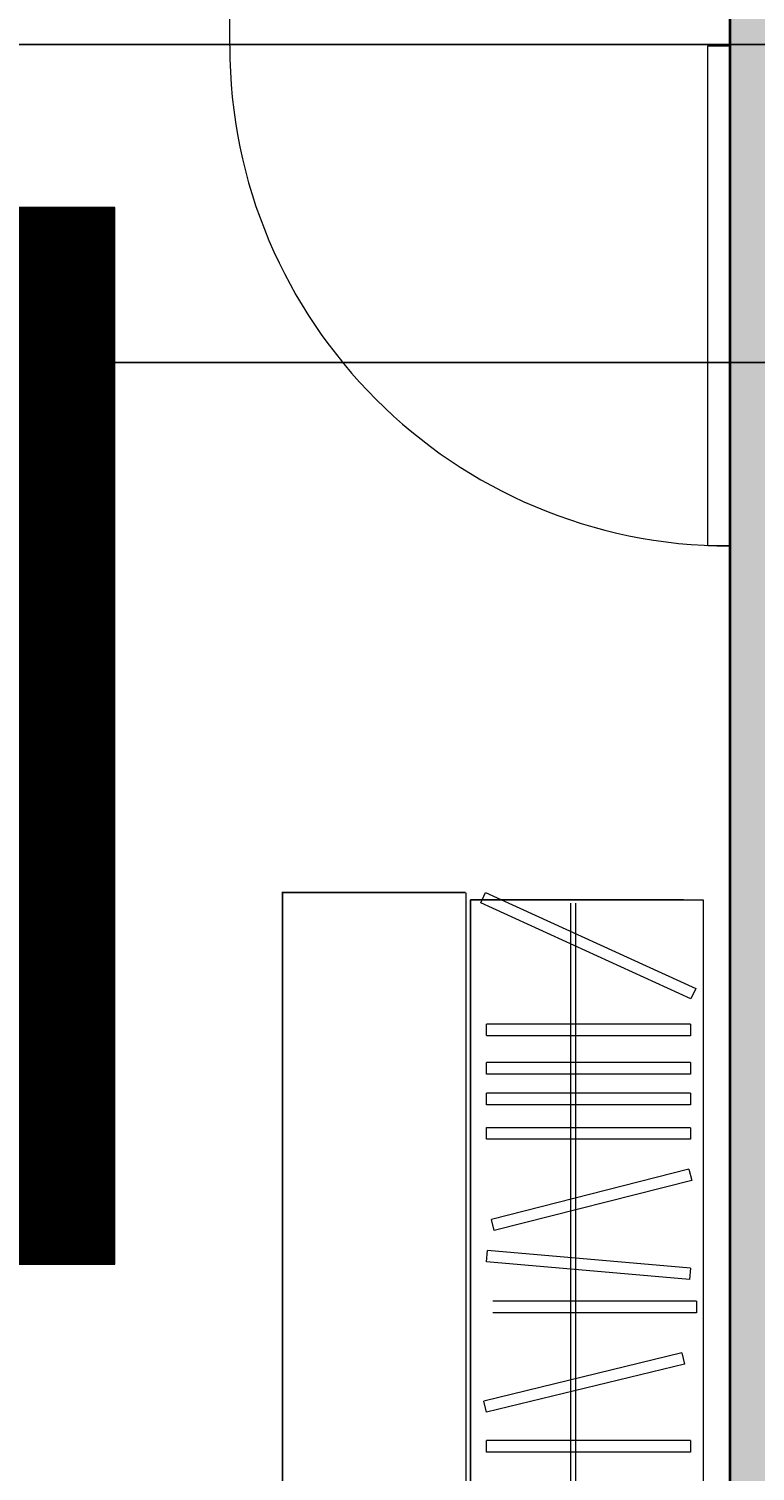
# Model space of a CAD drawing. Units: inches. Extents: x 192 to 1361, y -1362 to 367.
# Tile 9 of 23: x 495 to 649, y -761 to -454. Entities that reach past the tile are written whole.
import ezdxf

# ---------------------------------------------------------------- set-up
doc = ezdxf.new("R2010")
doc.units = ezdxf.units.IN
doc.header["$MEASUREMENT"] = 0
for name, color, linetype, lineweight in [('A-ANNO-DIMS', 2, 'Continuous', 18), ('A-DOOR', 4, 'Continuous', 18), ('A-FLOR', 8, 'Continuous', 18), ('A-WALL-PATT', 250, 'Continuous', 13), ('closet', 32, 'Continuous', 18), ('walls', 7, 'Continuous', 35)]:
    doc.layers.add(name, color=color, linetype=linetype, lineweight=lineweight)
doc.layers.add('A-FLOR-PATT', color=254, linetype='Continuous', lineweight=13, true_color=0xfeeab9)
doc.styles.get("Standard").update_dxf_attribs({"font": 'arial.ttf'})
doc.dimstyles.get("Standard").update_dxf_attribs({"dimtxt": 0.18, "dimasz": 0.18, "dimexe": 0.18, "dimexo": 0.0625, "dimgap": 0.09, "dimtad": 0, "dimtih": 1, "dimtoh": 1, "dimzin": 0, "dimdsep": 46, "dimlunit": 3, "dimtxsty": 'Standard', "dimcen": 0.09, "dimadec": 0, "dimazin": 0, "dimtfac": 1, "dimtofl": 0, "dimtmove": 0, "dimatfit": 3, "dimfxl": 1, "dimtolj": 1, "dimtzin": 0, "dimarcsym": 0})

# ---------------------------------------------------------------- blocks, each defined once
blk = doc.blocks.new('*U2')
for p, q in [((0, 0), (0, -6)), ((40, 0), (40, -6))]:
    blk.add_line(p, q)
blk.add_lwpolyline([(0, 0), (0, 40), (1.75, 40), (1.75, 0)], close=True)
blk.add_arc((0, 0), 40, 0, 90)
blk = doc.blocks.new('closet')
at = {"layer": 'closet'}
for p, q in [((-0.712, -5.577), (5.592, 8.191)), ((6.268, 7.882), (-0.036, -5.886)), ((5.592, 8.191), (6.268, 7.882)), ((7.922, 7.842), (8.679, 7.842)), ((7.922, 7.842), (7.922, -5.515)), ((8.679, 7.842), (8.679, -5.515)), ((10.443, 7.842), (11.2, 7.842)), ((10.443, 7.842), (10.443, -5.515)), ((11.2, 7.842), (11.2, -5.515)), ((12.449, 7.842), (13.206, 7.842)), ((12.449, 7.842), (12.449, -5.515)), ((13.206, 7.842), (13.206, -5.515)), ((14.712, 7.842), (15.469, 7.842)), ((14.712, 7.842), (14.712, -5.515)), ((15.469, 7.842), (15.469, -5.515)), ((17.436, 7.748), (18.17, 7.935)), ((17.436, 7.748), (20.729, -5.196)), ((18.17, 7.935), (21.462, -5.009)), ((23.918, 7.842), (22.755, -5.464)), ((24.672, 7.776), (23.509, -5.53)), ((23.918, 7.842), (24.672, 7.776)), ((26.086, 8.254), (26.086, -5.103)), ((26.843, 8.254), (26.843, -5.103)), ((35.229, 7.842), (35.229, -5.515)), ((35.986, 7.842), (35.986, -5.515)), ((40.326, 7.842), (40.326, -5.515)), ((41.083, 7.842), (41.083, -5.515)), ((42.848, 7.842), (42.848, -5.515)), ((43.605, 7.842), (43.605, -5.515)), ((45.896, 7.842), (45.896, -5.515)), ((46.653, 7.842), (46.653, -5.515)), ((50.066, 7.842), (50.066, -5.515)), ((50.823, 7.842), (50.823, -5.515)), ((53.325, 7.842), (53.325, -5.515)), ((54.081, 7.842), (54.081, -5.515)), ((55.896, 7.842), (55.896, -5.515)), ((56.653, 7.842), (56.653, -5.515)), ((57.994, -5.577), (64.297, 8.191)), ((64.973, 7.882), (58.669, -5.886)), ((60.189, -5.577), (66.493, 8.191)), ((67.169, 7.882), (60.865, -5.886)), ((61.999, -5.577), (68.303, 8.191)), ((68.978, 7.882), (62.675, -5.886)), ((69.963, 7.842), (69.963, -5.515)), ((70.72, 7.842), (70.72, -5.515)), ((72.429, 7.842), (72.429, -5.515)), ((73.186, 7.842), (73.186, -5.515)), ((74.817, 7.842), (74.817, -5.515)), ((75.574, 7.842), (75.574, -5.515)), ((76.936, 7.842), (76.936, -5.515)), ((77.693, 7.842), (77.693, -5.515)), ((-0.232, 7.394), (-0.232, -6.566)), ((29.485, 7.286), (32.636, -5.694)), ((30.221, 7.465), (33.372, -5.515)), ((56.234, 0.335), (0, 0.335)), ((56.2, 0), (0, 0)), ((56.2, 0), (78.757, 0)), ((56.234, 0.335), (78.757, 0.335)), ((-0.036, -5.886), (-0.712, -5.577)), ((21.462, -5.009), (20.729, -5.196)), ((23.509, -5.53), (22.755, -5.464)), ((33.372, -5.515), (32.636, -5.694)), ((35.986, -5.515), (35.229, -5.515)), ((41.083, -5.515), (40.326, -5.515)), ((43.605, -5.515), (42.848, -5.515)), ((46.653, -5.515), (45.896, -5.515)), ((50.823, -5.515), (50.066, -5.515)), ((54.081, -5.515), (53.325, -5.515)), ((56.653, -5.515), (55.896, -5.515)), ((58.669, -5.886), (57.994, -5.577)), ((60.865, -5.886), (60.189, -5.577)), ((62.675, -5.886), (61.999, -5.577)), ((70.72, -5.515), (69.963, -5.515)), ((73.186, -5.515), (72.429, -5.515)), ((75.574, -5.515), (74.817, -5.515)), ((77.693, -5.515), (76.936, -5.515))]:
    blk.add_line(p, q, dxfattribs=at)
blk = doc.blocks.new('rotated closet')
at = {"layer": 'closet'}
for p, q in [((26.318, 0.86), (27.074, 0.86)), ((29.717, -0.108), (30.452, 0.071)), ((35.461, 0.448), (36.217, 0.448)), ((40.558, 0.448), (41.314, 0.448)), ((43.08, 0.448), (43.837, 0.448)), ((46.128, 0.448), (46.884, 0.448)), ((50.298, 0.448), (51.055, 0.448)), ((53.556, 0.448), (54.313, 0.448)), ((56.128, 0.448), (56.884, 0.448)), ((64.529, 0.797), (65.205, 0.488)), ((66.725, 0.797), (67.4, 0.488)), ((68.534, 0.797), (69.21, 0.488)), ((70.195, 0.448), (70.952, 0.448)), ((72.66, 0.448), (73.417, 0.448)), ((75.049, 0.448), (75.806, 0.448)), ((77.168, 0.448), (77.924, 0.448)), ((78.989, 0), (78.989, -13.96)), ((8.91, -12.909), (8.153, -12.909)), ((11.431, -12.909), (10.675, -12.909)), ((13.437, -12.909), (12.681, -12.909)), ((15.7, -12.909), (14.943, -12.909)), ((0, -13.96), (78.989, -13.96)), ((-0.456, -14.274), (79.544, -14.274))]:
    blk.add_line(p, q, dxfattribs=at)
blk.add_blockref('closet', (0.232, -7.394), dxfattribs=at)
blk = doc.blocks.new('*D31')
at = {"layer": 'A-ANNO-DIMS', "color": 0, "lineweight": -2, "transparency": 16777216}
for p, q in [((587.7, -637.86), (548.65, -637.86)), ((548.83, -638.04), (548.83, -767.46)), ((548.83, -897.24), (548.83, -767.83)), ((587.7, -897.42), (548.65, -897.42))]:
    blk.add_line(p, q, dxfattribs=at)
at = {"layer": 'A-ANNO-DIMS', "color": 0, "transparency": 16777216}
for points in [[(548.8, -638.04), (548.86, -638.04), (548.83, -637.86)], [(548.8, -897.24), (548.86, -897.24), (548.83, -897.42)]]:
    blk.add_solid(points, dxfattribs=at)
at = {"layer": 'Defpoints', "color": 0, "transparency": 16777216}
for p in [(587.76, -637.86), (548.83, -897.42), (587.76, -897.42)]:
    blk.add_point(p, dxfattribs=at)
at = {"layer": 'A-ANNO-DIMS', "color": 0, "transparency": 16777216, "insert": (548.83, -767.64), "char_height": 0.18, "attachment_point": 5}
blk.add_mtext('\\A1;WARDROBE 260', dxfattribs=at)
blk = doc.blocks.new('*D69')
at = {"layer": 'A-ANNO-DIMS', "color": 0, "lineweight": -2, "transparency": 16777216}
for p, q in [((981.75, -457.5), (192.16, -457.5)), ((192.34, -457.68), (192.34, -491.13)), ((192.34, -524.95), (192.34, -491.5)), ((980.52, -525.13), (192.16, -525.13))]:
    blk.add_line(p, q, dxfattribs=at)
at = {"layer": 'A-ANNO-DIMS', "color": 0, "transparency": 16777216}
for points in [[(192.31, -457.68), (192.37, -457.68), (192.34, -457.5)], [(192.31, -524.95), (192.37, -524.95), (192.34, -525.13)]]:
    blk.add_solid(points, dxfattribs=at)
at = {"layer": 'Defpoints', "color": 0, "transparency": 16777216}
for p in [(981.81, -457.5), (192.34, -525.13), (980.58, -525.13)]:
    blk.add_point(p, dxfattribs=at)
at = {"layer": 'A-ANNO-DIMS', "color": 0, "transparency": 16777216, "insert": (192.34, -491.31), "char_height": 0.18, "attachment_point": 5}
blk.add_mtext('\\A1;67.63', dxfattribs=at)

msp = doc.modelspace()

# ---------------------------------------------------------------- hatches: boundary and pattern name
at = {"layer": 'A-FLOR-PATT'}
h = msp.add_hatch(dxfattribs=at)
h.set_pattern_fill('ANSI31', color=256)
edge = h.paths.add_edge_path()
edge.add_line((513.1511, -492.1899), (327.1032, -492.1899))
edge.add_line((327.1032, -492.1899), (327.1032, -508.439))
edge.add_line((327.1032, -508.439), (326.9465, -508.439))
edge.add_line((326.9465, -508.439), (326.6697, -537.1419))
edge.add_line((326.6697, -537.1419), (391.8439, -537.1419))
edge.add_line((391.8439, -537.1419), (391.8439, -520.2026))
edge.add_line((391.8439, -520.2026), (393.0084, -520.2026))
edge.add_spline(control_points=[(393.2858, -517.1545), (392.9584, -517.4172), (392.3119, -517.936), (392.9583, -518.8629), (393.4257, -519.6151), (393.1386, -520.0192), (393.0084, -520.2026)], knot_values=[0, 0, 0, 0, 0.65327829, 1.2901376, 1.74045698, 2.11445126, 2.11445126, 2.11445126, 2.11445126], degree=3, periodic=0)
edge.add_line((393.0084, -520.2026), (395.1098, -520.2026))
edge.add_spline(control_points=[(395.3872, -517.1545), (395.0598, -517.4172), (394.4133, -517.936), (395.0598, -518.8629), (395.5272, -519.6151), (395.2401, -520.0192), (395.1098, -520.2026)], knot_values=[0, 0, 0, 0, 0.65327829, 1.2901376, 1.74045698, 2.11445126, 2.11445126, 2.11445126, 2.11445126], degree=3, periodic=0)
edge.add_line((395.1098, -520.2026), (397.3144, -520.2026))
edge.add_spline(control_points=[(397.5918, -517.1545), (397.2644, -517.4172), (396.6179, -517.936), (397.2643, -518.8629), (397.7317, -519.6151), (397.4446, -520.0192), (397.3144, -520.2026)], knot_values=[0, 0, 0, 0, 0.65327829, 1.2901376, 1.74045698, 2.11445126, 2.11445126, 2.11445126, 2.11445126], degree=3, periodic=0)
edge.add_line((397.3144, -520.2026), (399.2806, -520.2026))
edge.add_spline(control_points=[(399.558, -517.1545), (399.2307, -517.4172), (398.5841, -517.936), (399.2306, -518.8629), (399.698, -519.6151), (399.4109, -520.0192), (399.2806, -520.2026)], knot_values=[0, 0, 0, 0, 0.65327829, 1.2901376, 1.74045698, 2.11445126, 2.11445126, 2.11445126, 2.11445126], degree=3, periodic=0)
edge.add_line((399.2806, -520.2026), (401.664, -520.2026))
edge.add_spline(control_points=[(401.9414, -517.1545), (401.614, -517.4172), (400.9675, -517.936), (401.6139, -518.8629), (402.0814, -519.6151), (401.7943, -520.0192), (401.664, -520.2026)], knot_values=[0, 0, 0, 0, 0.65327829, 1.2901376, 1.74045698, 2.11445126, 2.11445126, 2.11445126, 2.11445126], degree=3, periodic=0)
edge.add_line((401.664, -520.2026), (403.6961, -520.2026))
edge.add_spline(control_points=[(403.9735, -517.1545), (403.6461, -517.4172), (402.9996, -517.936), (403.6461, -518.8629), (404.1135, -519.6151), (403.8264, -520.0192), (403.6961, -520.2026)], knot_values=[0, 0, 0, 0, 0.65327829, 1.2901376, 1.74045698, 2.11445126, 2.11445126, 2.11445126, 2.11445126], degree=3, periodic=0)
edge.add_line((403.6961, -520.2026), (405.6624, -520.2026))
edge.add_spline(control_points=[(405.9398, -517.1545), (405.6124, -517.4172), (404.9659, -517.936), (405.6123, -518.8629), (406.0797, -519.6151), (405.7926, -520.0192), (405.6624, -520.2026)], knot_values=[0, 0, 0, 0, 0.65327829, 1.2901376, 1.74045698, 2.11445126, 2.11445126, 2.11445126, 2.11445126], degree=3, periodic=0)
edge.add_line((405.6624, -520.2026), (408.0457, -520.2026))
edge.add_spline(control_points=[(408.3231, -517.1545), (407.9958, -517.4172), (407.3493, -517.936), (407.9957, -518.8629), (408.4631, -519.6151), (408.176, -520.0192), (408.0457, -520.2026)], knot_values=[0, 0, 0, 0, 0.65327829, 1.2901376, 1.74045698, 2.11445126, 2.11445126, 2.11445126, 2.11445126], degree=3, periodic=0)
edge.add_line((408.0457, -520.2026), (410.8462, -520.2026))
edge.add_spline(control_points=[(411.1236, -517.1545), (410.7962, -517.4172), (410.1497, -517.936), (410.7961, -518.8629), (411.2635, -519.6151), (410.9764, -520.0192), (410.8462, -520.2026)], knot_values=[0, 0, 0, 0, 0.65327829, 1.2901376, 1.74045698, 2.11445126, 2.11445126, 2.11445126, 2.11445126], degree=3, periodic=0)
edge.add_line((410.8462, -520.2026), (413.2295, -520.2026))
edge.add_spline(control_points=[(413.5069, -517.1545), (413.1795, -517.4172), (412.533, -517.936), (413.1794, -518.8629), (413.6468, -519.6151), (413.3597, -520.0192), (413.2295, -520.2026)], knot_values=[0, 0, 0, 0, 0.65327829, 1.2901376, 1.74045698, 2.11445126, 2.11445126, 2.11445126, 2.11445126], degree=3, periodic=0)
edge.add_line((413.2295, -520.2026), (415.434, -520.2026))
edge.add_spline(control_points=[(415.7114, -517.1545), (415.3841, -517.4172), (414.7376, -517.936), (415.384, -518.8629), (415.8514, -519.6151), (415.5643, -520.0192), (415.434, -520.2026)], knot_values=[0, 0, 0, 0, 0.65327829, 1.2901376, 1.74045698, 2.11445126, 2.11445126, 2.11445126, 2.11445126], degree=3, periodic=0)
edge.add_line((415.434, -520.2026), (417.5321, -520.2026))
edge.add_spline(control_points=[(417.8095, -517.1545), (417.4821, -517.4172), (416.8356, -517.936), (417.482, -518.8629), (417.9494, -519.6151), (417.6623, -520.0192), (417.5321, -520.2026)], knot_values=[0, 0, 0, 0, 0.65327829, 1.2901376, 1.74045698, 2.11445126, 2.11445126, 2.11445126, 2.11445126], degree=3, periodic=0)
edge.add_line((417.5321, -520.2026), (419.7366, -520.2026))
edge.add_spline(control_points=[(420.014, -517.1545), (419.6867, -517.4172), (419.0401, -517.936), (419.6866, -518.8629), (420.154, -519.6151), (419.8669, -520.0192), (419.7366, -520.2026)], knot_values=[0, 0, 0, 0, 0.65327829, 1.2901376, 1.74045698, 2.11445126, 2.11445126, 2.11445126, 2.11445126], degree=3, periodic=0)
edge.add_line((419.7366, -520.2026), (421.7029, -520.2026))
edge.add_spline(control_points=[(421.9803, -517.1545), (421.6529, -517.4172), (421.0064, -517.936), (421.6528, -518.8629), (422.1202, -519.6151), (421.8331, -520.0192), (421.7029, -520.2026)], knot_values=[0, 0, 0, 0, 0.65327829, 1.2901376, 1.74045698, 2.11445126, 2.11445126, 2.11445126, 2.11445126], degree=3, periodic=0)
edge.add_line((421.7029, -520.2026), (424.0863, -520.2026))
edge.add_spline(control_points=[(424.3637, -517.1545), (424.0363, -517.4172), (423.3898, -517.936), (424.0362, -518.8629), (424.5036, -519.6151), (424.2165, -520.0192), (424.0863, -520.2026)], knot_values=[0, 0, 0, 0, 0.65327829, 1.2901376, 1.74045698, 2.11445126, 2.11445126, 2.11445126, 2.11445126], degree=3, periodic=0)
edge.add_line((424.0863, -520.2026), (426.1184, -520.2026))
edge.add_spline(control_points=[(426.3958, -517.1545), (426.0684, -517.4172), (425.4219, -517.936), (426.0683, -518.8629), (426.5357, -519.6151), (426.2486, -520.0192), (426.1184, -520.2026)], knot_values=[0, 0, 0, 0, 0.65327829, 1.2901376, 1.74045698, 2.11445126, 2.11445126, 2.11445126, 2.11445126], degree=3, periodic=0)
edge.add_line((426.1184, -520.2026), (428.0846, -520.2026))
edge.add_spline(control_points=[(428.362, -517.1545), (428.0346, -517.4172), (427.3881, -517.936), (428.0346, -518.8629), (428.502, -519.6151), (428.2149, -520.0192), (428.0846, -520.2026)], knot_values=[0, 0, 0, 0, 0.65327829, 1.2901376, 1.74045698, 2.11445126, 2.11445126, 2.11445126, 2.11445126], degree=3, periodic=0)
edge.add_line((428.0846, -520.2026), (430.468, -520.2026))
edge.add_spline(control_points=[(430.7454, -517.1545), (430.418, -517.4172), (429.7715, -517.936), (430.4179, -518.8629), (430.8853, -519.6151), (430.5983, -520.0192), (430.468, -520.2026)], knot_values=[0, 0, 0, 0, 0.65327829, 1.2901376, 1.74045698, 2.11445126, 2.11445126, 2.11445126, 2.11445126], degree=3, periodic=0)
edge.add_line((430.468, -520.2026), (433.2684, -520.2026))
edge.add_spline(control_points=[(433.5458, -517.1545), (433.2184, -517.4172), (432.5719, -517.936), (433.2184, -518.8629), (433.6858, -519.6151), (433.3987, -520.0192), (433.2684, -520.2026)], knot_values=[0, 0, 0, 0, 0.65327829, 1.2901376, 1.74045698, 2.11445126, 2.11445126, 2.11445126, 2.11445126], degree=3, periodic=0)
edge.add_line((433.2684, -520.2026), (435.6517, -520.2026))
edge.add_spline(control_points=[(435.9291, -517.1545), (435.6017, -517.4172), (434.9552, -517.936), (435.6017, -518.8629), (436.0691, -519.6151), (435.782, -520.0192), (435.6517, -520.2026)], knot_values=[0, 0, 0, 0, 0.65327829, 1.2901376, 1.74045698, 2.11445126, 2.11445126, 2.11445126, 2.11445126], degree=3, periodic=0)
edge.add_line((435.6517, -520.2026), (437.8563, -520.2026))
edge.add_spline(control_points=[(438.1337, -517.1545), (437.8063, -517.4172), (437.1598, -517.936), (437.8062, -518.8629), (438.2736, -519.6151), (437.9865, -520.0192), (437.8563, -520.2026)], knot_values=[0, 0, 0, 0, 0.65327829, 1.2901376, 1.74045698, 2.11445126, 2.11445126, 2.11445126, 2.11445126], degree=3, periodic=0)
edge.add_line((437.8563, -520.2026), (439.7189, -520.2026))
edge.add_spline(control_points=[(439.9963, -517.1545), (439.669, -517.4172), (439.0225, -517.936), (439.6689, -518.8629), (440.1363, -519.6151), (439.8492, -520.0192), (439.7189, -520.2026)], knot_values=[0, 0, 0, 0, 0.65327829, 1.2901376, 1.74045698, 2.11445126, 2.11445126, 2.11445126, 2.11445126], degree=3, periodic=0)
edge.add_line((439.7189, -520.2026), (441.9235, -520.2026))
edge.add_spline(control_points=[(442.2009, -517.1545), (441.8735, -517.4172), (441.227, -517.936), (441.8735, -518.8629), (442.3409, -519.6151), (442.0538, -520.0192), (441.9235, -520.2026)], knot_values=[0, 0, 0, 0, 0.65327829, 1.2901376, 1.74045698, 2.11445126, 2.11445126, 2.11445126, 2.11445126], degree=3, periodic=0)
edge.add_line((441.9235, -520.2026), (443.8898, -520.2026))
edge.add_spline(control_points=[(444.1672, -517.1545), (443.8398, -517.4172), (443.1933, -517.936), (443.8397, -518.8629), (444.3071, -519.6151), (444.02, -520.0192), (443.8898, -520.2026)], knot_values=[0, 0, 0, 0, 0.65327829, 1.2901376, 1.74045698, 2.11445126, 2.11445126, 2.11445126, 2.11445126], degree=3, periodic=0)
edge.add_line((443.8898, -520.2026), (446.2731, -520.2026))
edge.add_spline(control_points=[(446.5505, -517.1545), (446.2232, -517.4172), (445.5767, -517.936), (446.2231, -518.8629), (446.6905, -519.6151), (446.4034, -520.0192), (446.2731, -520.2026)], knot_values=[0, 0, 0, 0, 0.65327829, 1.2901376, 1.74045698, 2.11445126, 2.11445126, 2.11445126, 2.11445126], degree=3, periodic=0)
edge.add_line((446.2731, -520.2026), (448.3052, -520.2026))
edge.add_spline(control_points=[(448.5826, -517.1545), (448.2553, -517.4172), (447.6088, -517.936), (448.2552, -518.8629), (448.7226, -519.6151), (448.4355, -520.0192), (448.3052, -520.2026)], knot_values=[0, 0, 0, 0, 0.65327829, 1.2901376, 1.74045698, 2.11445126, 2.11445126, 2.11445126, 2.11445126], degree=3, periodic=0)
edge.add_line((448.3052, -520.2026), (450.2715, -520.2026))
edge.add_spline(control_points=[(450.5489, -517.1545), (450.2215, -517.4172), (449.575, -517.936), (450.2214, -518.8629), (450.6888, -519.6151), (450.4018, -520.0192), (450.2715, -520.2026)], knot_values=[0, 0, 0, 0, 0.65327829, 1.2901376, 1.74045698, 2.11445126, 2.11445126, 2.11445126, 2.11445126], degree=3, periodic=0)
edge.add_line((450.2715, -520.2026), (452.6549, -520.2026))
edge.add_spline(control_points=[(452.9323, -517.1545), (452.6049, -517.4172), (451.9584, -517.936), (452.6048, -518.8629), (453.0722, -519.6151), (452.7851, -520.0192), (452.6549, -520.2026)], knot_values=[0, 0, 0, 0, 0.65327829, 1.2901376, 1.74045698, 2.11445126, 2.11445126, 2.11445126, 2.11445126], degree=3, periodic=0)
edge.add_line((452.6549, -520.2026), (453.8151, -520.2026))
edge.add_spline(control_points=[(454.0925, -517.1545), (453.7499, -517.417), (453.0754, -517.9338), (453.769, -518.8576), (454.2314, -519.6154), (453.945, -520.0193), (453.8151, -520.2026)], knot_values=[0, 0, 0, 0, 0.6639037, 1.30740562, 1.757725, 2.13171928, 2.13171928, 2.13171928, 2.13171928], degree=3, periodic=0)
edge.add_line((453.8151, -520.2026), (455.3467, -520.2026))
edge.add_spline(control_points=[(455.6241, -517.1545), (455.2967, -517.4172), (454.6502, -517.936), (455.2967, -518.8629), (455.7641, -519.6151), (455.477, -520.0192), (455.3467, -520.2026)], knot_values=[0, 0, 0, 0, 0.65327829, 1.2901376, 1.74045698, 2.11445126, 2.11445126, 2.11445126, 2.11445126], degree=3, periodic=0)
edge.add_line((455.3467, -520.2026), (456.895, -520.2026))
edge.add_spline(control_points=[(456.895, -520.2026), (457.0253, -520.0192), (457.3124, -519.6151), (456.845, -518.8629), (456.1986, -517.936), (456.8451, -517.4172), (457.1724, -517.1545)], knot_values=[0, 0, 0, 0, 0.37399428, 0.82431366, 1.46117297, 2.11445126, 2.11445126, 2.11445126, 2.11445126], degree=3, periodic=0)
edge.add_spline(control_points=[(458.0074, -517.1545), (457.68, -517.4172), (457.0335, -517.936), (457.68, -518.8629), (458.1474, -519.6151), (457.8603, -520.0192), (457.73, -520.2026)], knot_values=[0, 0, 0, 0, 0.65327829, 1.2901376, 1.74045698, 2.11445126, 2.11445126, 2.11445126, 2.11445126], degree=3, periodic=0)
edge.add_line((457.73, -520.2026), (458.8613, -520.2026))
edge.add_spline(control_points=[(459.1387, -517.1545), (458.8113, -517.4172), (458.1648, -517.936), (458.8112, -518.8629), (459.2786, -519.6151), (458.9916, -520.0192), (458.8613, -520.2026)], knot_values=[0, 0, 0, 0, 0.65327829, 1.2901376, 1.74045698, 2.11445126, 2.11445126, 2.11445126, 2.11445126], degree=3, periodic=0)
edge.add_line((458.8613, -520.2026), (459.9346, -520.2026))
edge.add_spline(control_points=[(460.212, -517.1545), (459.8846, -517.4172), (459.2381, -517.936), (459.8845, -518.8629), (460.3519, -519.6151), (460.0648, -520.0192), (459.9346, -520.2026)], knot_values=[0, 0, 0, 0, 0.65327829, 1.2901376, 1.74045698, 2.11445126, 2.11445126, 2.11445126, 2.11445126], degree=3, periodic=0)
edge.add_line((459.9346, -520.2026), (461.2447, -520.2026))
edge.add_spline(control_points=[(461.5221, -517.1545), (461.1947, -517.4172), (460.5482, -517.936), (461.1946, -518.8629), (461.662, -519.6151), (461.3749, -520.0192), (461.2447, -520.2026)], knot_values=[0, 0, 0, 0, 0.65327829, 1.2901376, 1.74045698, 2.11445126, 2.11445126, 2.11445126, 2.11445126], degree=3, periodic=0)
edge.add_line((461.2447, -520.2026), (462.6002, -520.2026))
edge.add_spline(control_points=[(462.8776, -517.1545), (462.5502, -517.4172), (461.9037, -517.936), (462.5501, -518.8629), (463.0175, -519.6151), (462.7304, -520.0192), (462.6002, -520.2026)], knot_values=[0, 0, 0, 0, 0.65327829, 1.2901376, 1.74045698, 2.11445126, 2.11445126, 2.11445126, 2.11445126], degree=3, periodic=0)
edge.add_line((462.6002, -520.2026), (463.0739, -520.2026))
edge.add_line((463.0739, -520.2026), (463.0739, -691.0271))
edge.add_line((463.0739, -691.0271), (462.6214, -691.0271))
edge.add_spline(control_points=[(462.8776, -694.0453), (462.5502, -693.7826), (461.9037, -693.2638), (462.5501, -692.3369), (463.011, -691.5951), (462.7443, -691.2005), (462.6214, -691.0271)], knot_values=[0, 0, 0, 0, 0.65327829, 1.2901376, 1.74045698, 2.09412198, 2.09412198, 2.09412198, 2.09412198], degree=3, periodic=0)
edge.add_line((462.6214, -691.0271), (461.3416, -691.0271))
edge.add_spline(control_points=[(461.5978, -694.0453), (461.2704, -693.7826), (460.6239, -693.2638), (461.2703, -692.3369), (461.7312, -691.5951), (461.4644, -691.2005), (461.3416, -691.0271)], knot_values=[0, 0, 0, 0, 0.65327829, 1.2901376, 1.74045698, 2.09412198, 2.09412198, 2.09412198, 2.09412198], degree=3, periodic=0)
edge.add_line((461.3416, -691.0271), (460.0315, -691.0271))
edge.add_spline(control_points=[(460.2877, -694.0453), (459.9603, -693.7826), (459.3138, -693.2638), (459.9602, -692.3369), (460.4211, -691.5951), (460.1544, -691.2005), (460.0315, -691.0271)], knot_values=[0, 0, 0, 0, 0.65327829, 1.2901376, 1.74045698, 2.09412198, 2.09412198, 2.09412198, 2.09412198], degree=3, periodic=0)
edge.add_line((460.0315, -691.0271), (458.9582, -691.0271))
edge.add_spline(control_points=[(459.2144, -694.0453), (458.887, -693.7826), (458.2405, -693.2638), (458.8869, -692.3369), (459.3478, -691.5951), (459.0811, -691.2005), (458.9582, -691.0271)], knot_values=[0, 0, 0, 0, 0.65327829, 1.2901376, 1.74045698, 2.09412198, 2.09412198, 2.09412198, 2.09412198], degree=3, periodic=0)
edge.add_line((458.9582, -691.0271), (457.8269, -691.0271))
edge.add_spline(control_points=[(457.8269, -691.0271), (457.9464, -691.2008), (458.2187, -691.5966), (457.7545, -692.3366), (457.1096, -693.2638), (457.7558, -693.7826), (458.0831, -694.0453)], knot_values=[0, 0, 0, 0, 0.3521435, 0.80246288, 1.43932219, 2.09260048, 2.09260048, 2.09260048, 2.09260048], degree=3, periodic=0)
edge.add_spline(control_points=[(457.2481, -694.0453), (456.9209, -693.7826), (456.2746, -693.2638), (456.9195, -692.3366), (457.3837, -691.5966), (457.1114, -691.2008), (456.992, -691.0271)], knot_values=[0, 0, 0, 0, 0.65327829, 1.2901376, 1.74045698, 2.09260048, 2.09260048, 2.09260048, 2.09260048], degree=3, periodic=0)
edge.add_line((456.992, -691.0271), (455.4436, -691.0271))
edge.add_spline(control_points=[(455.6998, -694.0453), (455.3725, -693.7826), (454.7263, -693.2638), (455.3712, -692.3366), (455.8354, -691.5966), (455.5631, -691.2008), (455.4436, -691.0271)], knot_values=[0, 0, 0, 0, 0.65327829, 1.2901376, 1.74045698, 2.09260048, 2.09260048, 2.09260048, 2.09260048], degree=3, periodic=0)
edge.add_line((455.4436, -691.0271), (453.8363, -691.0271))
edge.add_spline(control_points=[(454.0925, -694.0453), (453.7602, -693.7827), (453.1046, -693.2646), (453.7653, -692.3383), (454.2277, -691.5965), (453.9557, -691.2008), (453.8363, -691.0271)], knot_values=[0, 0, 0, 0, 0.65679228, 1.29582582, 1.7461452, 2.0982924, 2.0982924, 2.0982924, 2.0982924], degree=3, periodic=0)
edge.add_line((453.8363, -691.0271), (452.6761, -691.0271))
edge.add_spline(control_points=[(452.9323, -694.0453), (452.605, -693.7826), (451.9587, -693.2638), (452.6037, -692.3366), (453.0678, -691.5966), (452.7956, -691.2008), (452.6761, -691.0271)], knot_values=[0, 0, 0, 0, 0.65327829, 1.2901376, 1.74045698, 2.09260048, 2.09260048, 2.09260048, 2.09260048], degree=3, periodic=0)
edge.add_line((452.6761, -691.0271), (450.2927, -691.0271))
edge.add_spline(control_points=[(450.5489, -694.0453), (450.2216, -693.7826), (449.5753, -693.2638), (450.2203, -692.3366), (450.6845, -691.5966), (450.4122, -691.2008), (450.2927, -691.0271)], knot_values=[0, 0, 0, 0, 0.65327829, 1.2901376, 1.74045698, 2.09260048, 2.09260048, 2.09260048, 2.09260048], degree=3, periodic=0)
edge.add_line((450.2927, -691.0271), (448.3265, -691.0271))
edge.add_spline(control_points=[(448.5826, -694.0453), (448.2553, -693.7826), (447.6088, -693.2638), (448.2552, -692.3369), (448.7161, -691.5951), (448.4493, -691.2005), (448.3265, -691.0271)], knot_values=[0, 0, 0, 0, 0.65327829, 1.2901376, 1.74045698, 2.09412198, 2.09412198, 2.09412198, 2.09412198], degree=3, periodic=0)
edge.add_line((448.3265, -691.0271), (446.2944, -691.0271))
edge.add_spline(control_points=[(446.5505, -694.0453), (446.2232, -693.7826), (445.5767, -693.2638), (446.2231, -692.3369), (446.684, -691.5951), (446.4172, -691.2005), (446.2944, -691.0271)], knot_values=[0, 0, 0, 0, 0.65327829, 1.2901376, 1.74045698, 2.09412198, 2.09412198, 2.09412198, 2.09412198], degree=3, periodic=0)
edge.add_line((446.2944, -691.0271), (443.911, -691.0271))
edge.add_spline(control_points=[(444.1672, -694.0453), (443.8398, -693.7826), (443.1933, -693.2638), (443.8397, -692.3369), (444.3006, -691.5951), (444.0338, -691.2005), (443.911, -691.0271)], knot_values=[0, 0, 0, 0, 0.65327829, 1.2901376, 1.74045698, 2.09412198, 2.09412198, 2.09412198, 2.09412198], degree=3, periodic=0)
edge.add_line((443.911, -691.0271), (441.9447, -691.0271))
edge.add_spline(control_points=[(442.2009, -694.0453), (441.8735, -693.7826), (441.227, -693.2638), (441.8735, -692.3369), (442.3344, -691.5951), (442.0676, -691.2005), (441.9447, -691.0271)], knot_values=[0, 0, 0, 0, 0.65327829, 1.2901376, 1.74045698, 2.09412198, 2.09412198, 2.09412198, 2.09412198], degree=3, periodic=0)
edge.add_line((441.9447, -691.0271), (439.7402, -691.0271))
edge.add_spline(control_points=[(439.9963, -694.0453), (439.669, -693.7826), (439.0225, -693.2638), (439.6689, -692.3369), (440.1298, -691.5951), (439.863, -691.2005), (439.7402, -691.0271)], knot_values=[0, 0, 0, 0, 0.65327829, 1.2901376, 1.74045698, 2.09412198, 2.09412198, 2.09412198, 2.09412198], degree=3, periodic=0)
edge.add_line((439.7402, -691.0271), (437.8775, -691.0271))
edge.add_spline(control_points=[(438.1337, -694.0453), (437.8063, -693.7826), (437.1598, -693.2638), (437.8062, -692.3369), (438.2671, -691.5951), (438.0004, -691.2005), (437.8775, -691.0271)], knot_values=[0, 0, 0, 0, 0.65327829, 1.2901376, 1.74045698, 2.09412198, 2.09412198, 2.09412198, 2.09412198], degree=3, periodic=0)
edge.add_line((437.8775, -691.0271), (435.6729, -691.0271))
edge.add_spline(control_points=[(435.9291, -694.0453), (435.6017, -693.7826), (434.9552, -693.2638), (435.6017, -692.3369), (436.0626, -691.5951), (435.7958, -691.2005), (435.6729, -691.0271)], knot_values=[0, 0, 0, 0, 0.65327829, 1.2901376, 1.74045698, 2.09412198, 2.09412198, 2.09412198, 2.09412198], degree=3, periodic=0)
edge.add_line((435.6729, -691.0271), (433.2896, -691.0271))
edge.add_spline(control_points=[(433.5458, -694.0453), (433.2184, -693.7826), (432.5719, -693.2638), (433.2184, -692.3369), (433.6793, -691.5951), (433.4125, -691.2005), (433.2896, -691.0271)], knot_values=[0, 0, 0, 0, 0.65327829, 1.2901376, 1.74045698, 2.09412198, 2.09412198, 2.09412198, 2.09412198], degree=3, periodic=0)
edge.add_line((433.2896, -691.0271), (430.4892, -691.0271))
edge.add_spline(control_points=[(430.7454, -694.0453), (430.418, -693.7826), (429.7715, -693.2638), (430.4179, -692.3369), (430.8788, -691.5951), (430.6121, -691.2005), (430.4892, -691.0271)], knot_values=[0, 0, 0, 0, 0.65327829, 1.2901376, 1.74045698, 2.09412198, 2.09412198, 2.09412198, 2.09412198], degree=3, periodic=0)
edge.add_line((430.4892, -691.0271), (428.1058, -691.0271))
edge.add_spline(control_points=[(428.362, -694.0453), (428.0346, -693.7826), (427.3881, -693.2638), (428.0346, -692.3369), (428.4955, -691.5951), (428.2287, -691.2005), (428.1058, -691.0271)], knot_values=[0, 0, 0, 0, 0.65327829, 1.2901376, 1.74045698, 2.09412198, 2.09412198, 2.09412198, 2.09412198], degree=3, periodic=0)
edge.add_line((428.1058, -691.0271), (426.1396, -691.0271))
edge.add_spline(control_points=[(426.3958, -694.0453), (426.0684, -693.7826), (425.4219, -693.2638), (426.0683, -692.3369), (426.5292, -691.5951), (426.2624, -691.2005), (426.1396, -691.0271)], knot_values=[0, 0, 0, 0, 0.65327829, 1.2901376, 1.74045698, 2.09412198, 2.09412198, 2.09412198, 2.09412198], degree=3, periodic=0)
edge.add_line((426.1396, -691.0271), (424.1075, -691.0271))
edge.add_spline(control_points=[(424.3637, -694.0453), (424.0363, -693.7826), (423.3898, -693.2638), (424.0362, -692.3369), (424.4971, -691.5951), (424.2303, -691.2005), (424.1075, -691.0271)], knot_values=[0, 0, 0, 0, 0.65327829, 1.2901376, 1.74045698, 2.09412198, 2.09412198, 2.09412198, 2.09412198], degree=3, periodic=0)
edge.add_line((424.1075, -691.0271), (421.7241, -691.0271))
edge.add_spline(control_points=[(421.9803, -694.0453), (421.6529, -693.7826), (421.0064, -693.2638), (421.6528, -692.3369), (422.1137, -691.5951), (421.847, -691.2005), (421.7241, -691.0271)], knot_values=[0, 0, 0, 0, 0.65327829, 1.2901376, 1.74045698, 2.09412198, 2.09412198, 2.09412198, 2.09412198], degree=3, periodic=0)
edge.add_line((421.7241, -691.0271), (419.7579, -691.0271))
edge.add_spline(control_points=[(420.014, -694.0453), (419.6867, -693.7826), (419.0401, -693.2638), (419.6866, -692.3369), (420.1475, -691.5951), (419.8807, -691.2005), (419.7579, -691.0271)], knot_values=[0, 0, 0, 0, 0.65327829, 1.2901376, 1.74045698, 2.09412198, 2.09412198, 2.09412198, 2.09412198], degree=3, periodic=0)
edge.add_line((419.7579, -691.0271), (417.5533, -691.0271))
edge.add_spline(control_points=[(417.8095, -694.0453), (417.4821, -693.7826), (416.8356, -693.2638), (417.482, -692.3369), (417.9429, -691.5951), (417.6761, -691.2005), (417.5533, -691.0271)], knot_values=[0, 0, 0, 0, 0.65327829, 1.2901376, 1.74045698, 2.09412198, 2.09412198, 2.09412198, 2.09412198], degree=3, periodic=0)
edge.add_line((417.5533, -691.0271), (415.4553, -691.0271))
edge.add_spline(control_points=[(415.7114, -694.0453), (415.3841, -693.7826), (414.7376, -693.2638), (415.384, -692.3369), (415.8449, -691.5951), (415.5781, -691.2005), (415.4553, -691.0271)], knot_values=[0, 0, 0, 0, 0.65327829, 1.2901376, 1.74045698, 2.09412198, 2.09412198, 2.09412198, 2.09412198], degree=3, periodic=0)
edge.add_line((415.4553, -691.0271), (413.2507, -691.0271))
edge.add_spline(control_points=[(413.5069, -694.0453), (413.1795, -693.7826), (412.533, -693.2638), (413.1794, -692.3369), (413.6403, -691.5951), (413.3736, -691.2005), (413.2507, -691.0271)], knot_values=[0, 0, 0, 0, 0.65327829, 1.2901376, 1.74045698, 2.09412198, 2.09412198, 2.09412198, 2.09412198], degree=3, periodic=0)
edge.add_line((413.2507, -691.0271), (410.8674, -691.0271))
edge.add_spline(control_points=[(411.1236, -694.0453), (410.7962, -693.7826), (410.1497, -693.2638), (410.7961, -692.3369), (411.257, -691.5951), (410.9903, -691.2005), (410.8674, -691.0271)], knot_values=[0, 0, 0, 0, 0.65327829, 1.2901376, 1.74045698, 2.09412198, 2.09412198, 2.09412198, 2.09412198], degree=3, periodic=0)
edge.add_line((410.8674, -691.0271), (408.067, -691.0271))
edge.add_spline(control_points=[(408.3231, -694.0453), (407.9958, -693.7826), (407.3493, -693.2638), (407.9957, -692.3369), (408.4566, -691.5951), (408.1898, -691.2005), (408.067, -691.0271)], knot_values=[0, 0, 0, 0, 0.65327829, 1.2901376, 1.74045698, 2.09412198, 2.09412198, 2.09412198, 2.09412198], degree=3, periodic=0)
edge.add_line((408.067, -691.0271), (405.6836, -691.0271))
edge.add_spline(control_points=[(405.9398, -694.0453), (405.6124, -693.7826), (404.9659, -693.2638), (405.6123, -692.3369), (406.0732, -691.5951), (405.8064, -691.2005), (405.6836, -691.0271)], knot_values=[0, 0, 0, 0, 0.65327829, 1.2901376, 1.74045698, 2.09412198, 2.09412198, 2.09412198, 2.09412198], degree=3, periodic=0)
edge.add_line((405.6836, -691.0271), (403.7173, -691.0271))
edge.add_spline(control_points=[(403.9735, -694.0453), (403.6461, -693.7826), (402.9996, -693.2638), (403.6461, -692.3369), (404.107, -691.5951), (403.8402, -691.2005), (403.7173, -691.0271)], knot_values=[0, 0, 0, 0, 0.65327829, 1.2901376, 1.74045698, 2.09412198, 2.09412198, 2.09412198, 2.09412198], degree=3, periodic=0)
edge.add_line((403.7173, -691.0271), (401.6852, -691.0271))
edge.add_spline(control_points=[(401.9414, -694.0453), (401.614, -693.7826), (400.9675, -693.2638), (401.6139, -692.3369), (402.0749, -691.5951), (401.8081, -691.2005), (401.6852, -691.0271)], knot_values=[0, 0, 0, 0, 0.65327829, 1.2901376, 1.74045698, 2.09412198, 2.09412198, 2.09412198, 2.09412198], degree=3, periodic=0)
edge.add_line((401.6852, -691.0271), (399.3019, -691.0271))
edge.add_spline(control_points=[(399.558, -694.0453), (399.2307, -693.7826), (398.5841, -693.2638), (399.2306, -692.3369), (399.6915, -691.5951), (399.4247, -691.2005), (399.3019, -691.0271)], knot_values=[0, 0, 0, 0, 0.65327829, 1.2901376, 1.74045698, 2.09412198, 2.09412198, 2.09412198, 2.09412198], degree=3, periodic=0)
edge.add_line((399.3019, -691.0271), (397.3356, -691.0271))
edge.add_spline(control_points=[(397.5918, -694.0453), (397.2644, -693.7826), (396.6179, -693.2638), (397.2643, -692.3369), (397.7252, -691.5951), (397.4585, -691.2005), (397.3356, -691.0271)], knot_values=[0, 0, 0, 0, 0.65327829, 1.2901376, 1.74045698, 2.09412198, 2.09412198, 2.09412198, 2.09412198], degree=3, periodic=0)
edge.add_line((397.3356, -691.0271), (395.131, -691.0271))
edge.add_spline(control_points=[(395.3872, -694.0453), (395.0598, -693.7826), (394.4133, -693.2638), (395.0598, -692.3369), (395.5207, -691.5951), (395.2539, -691.2005), (395.131, -691.0271)], knot_values=[0, 0, 0, 0, 0.65327829, 1.2901376, 1.74045698, 2.09412198, 2.09412198, 2.09412198, 2.09412198], degree=3, periodic=0)
edge.add_line((395.131, -691.0271), (393.0296, -691.0271))
edge.add_spline(control_points=[(393.2858, -694.0453), (392.9584, -693.7826), (392.3119, -693.2638), (392.9583, -692.3369), (393.4192, -691.5951), (393.1524, -691.2005), (393.0296, -691.0271)], knot_values=[0, 0, 0, 0, 0.65327829, 1.2901376, 1.74045698, 2.09412198, 2.09412198, 2.09412198, 2.09412198], degree=3, periodic=0)
edge.add_line((393.0296, -691.0271), (391.8439, -691.0271))
edge.add_line((391.8439, -691.0271), (391.8439, -665.2551))
edge.add_line((391.8439, -665.2551), (326.6697, -665.2551))
edge.add_line((326.6697, -665.2551), (326.3929, -693.958))
edge.add_line((326.3929, -693.958), (326.3929, -716.9381))
edge.add_line((326.3929, -716.9381), (513.1511, -716.9381))
edge.add_line((513.1511, -716.9381), (513.1511, -492.1899))
h.paths.add_polyline_path([(353.9763, -588.1534), (487.3258, -588.1534), (487.3258, -561.3965), (353.9763, -561.3965)], flags=25)
at = {"layer": 'A-WALL-PATT'}
h = msp.add_hatch(color=256, dxfattribs=at)
h.dxf.hatch_style = 1
h.paths.add_polyline_path([(652.8925, -441.898), (643.8925, -441.898), (643.8925, -457.8461), (643.8925, -564.167), (643.8925, -905.4415), (578.0245, -905.4415), (578.0245, -914.4415), (643.8925, -914.4415), (643.8925, -969.5484), (652.6138, -969.5484), (652.6138, -963.172), (652.6138, -914.556)])
h.paths.add_polyline_path([(509.5452, 191.102), (504.3983, 191.102), (504.3983, 182.102), (509.5452, 182.102)])

# ---------------------------------------------------------------- linework, layer by layer
at = {"layer": 'A-FLOR'}
for p, q in [((513.1511, -492.1899), (327.1032, -492.1899)), ((513.1511, -716.9381), (513.1511, -492.1899)), ((326.3929, -716.9381), (513.1511, -716.9381))]:
    msp.add_line(p, q, dxfattribs=at)
at = {"layer": 'closet'}
for p, q in [((587.7625, -637.9412), (587.7625, -897.4218)), ((588.7836, -639.4217), (634.0617, -639.4217)), ((588.7836, -895.6222), (588.7836, -639.4217)), ((634.0617, -639.4217), (638.256, -639.4217)), ((638.256, -639.4217), (638.256, -895.6222))]:
    msp.add_line(p, q, dxfattribs=at)
at = {"layer": 'walls'}
msp.add_line((643.8925, -441.898), (643.8925, -905.4415), dxfattribs=at)

# ---------------------------------------------------------------- block references
at = {"layer": 'A-DOOR', "xscale": 2.658020973626523, "yscale": 2.658020973626523, "zscale": 2.658020973626523, "rotation": 180}
msp.add_blockref('*U2', (643.8925, -457.8461), dxfattribs=at)
at = {"layer": 'closet', "xscale": 3.243507334136714, "yscale": 3.243507334136714, "zscale": 3.243507334136714, "rotation": 269.9999999992008}
msp.add_blockref('rotated closet', (634.0617, -639.4217), dxfattribs=at)

# ---------------------------------------------------------------- dimensions: what is measured, and where the dimension line sits
at = {"layer": 'A-ANNO-DIMS'}
dim = msp.add_linear_dim(base=(192.3425, -525.128), p1=(981.8078, -457.4996), p2=(980.5799, -525.128), angle=90, dimstyle='Standard', override={"dimdec": 2, "dimlfac": 1, "dimrnd": 0, "dimzin": 0, "dimdsep": 46, "dimlunit": 2}, dxfattribs=at)
dim.commit()
dim.dimension.update_dxf_attribs({"geometry": '*D69', "text_midpoint": (192.3425, -491.3138)})
dim = msp.add_linear_dim(base=(548.8289, -897.4218), p1=(587.7625, -637.8641), p2=(587.7625, -897.4218), angle=270, text='WARDROBE <>', dimstyle='Standard', override={"dimdec": 0, "dimlfac": 1, "dimrnd": 0, "dimzin": 0, "dimdsep": 46, "dimlunit": 2}, dxfattribs=at)
dim.commit()
dim.dimension.update_dxf_attribs({"geometry": '*D31', "text_midpoint": (548.8289, -767.6429)})

doc.saveas('drawing.dxf')
